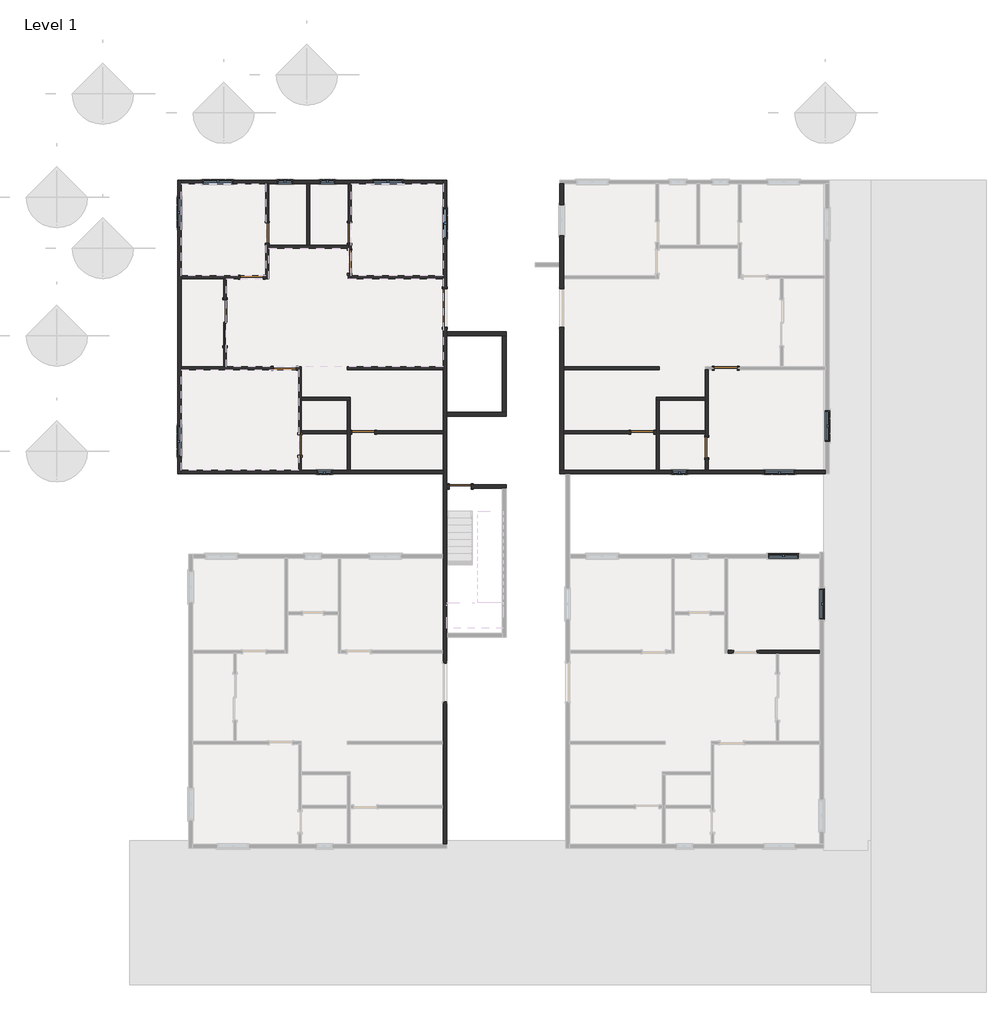
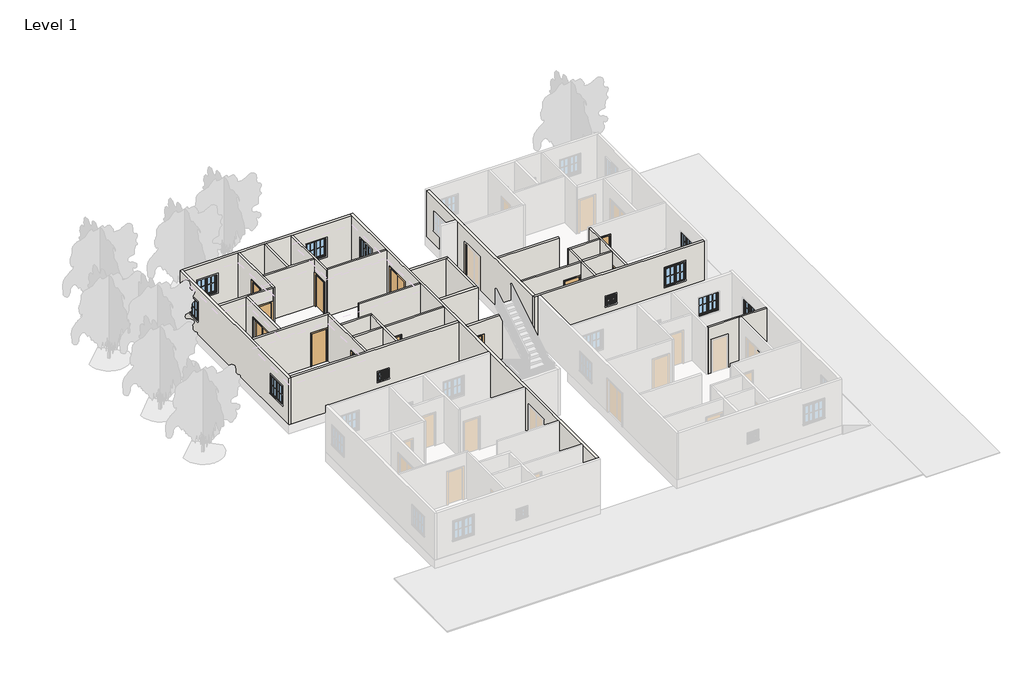
# One storey, part 2 of 7: 29 walls, 13 doors, 13 windows.
"""IFC4 building model written with IfcOpenShell, lengths in millimetres."""

from ifc_helpers import new_model, si_unit, frame, origin, origin_with_axes, place, context, project, spatial, polyline, outline, extrude, faceted_brep, transform, mapped, element, save
from components import door_a09c2f77, door_166d4031, door_d141acb4, door_b6e9fca3, door_e5f9f3c4, window_0c121b81, window_191d0cfb

model = new_model("IFC4")

# Units and contexts
model_context = context("Model", 3, world=origin())
ifc_project = project(units=[si_unit("LENGTHUNIT", "METRE", prefix="MILLI")], contexts=[model_context])

# Site, building, storey
site = spatial("IfcSite", under=ifc_project)
building = spatial("IfcBuilding", under=site)
storey = spatial("IfcBuildingStorey", under=building, Name="Level 1", Elevation=0.0)

# Doors
placement = place(None, origin())
door_shape = door_a09c2f77(model_context)
element("IfcDoor", 1, ObjectType="Door-Double-Flush_Panel : 60\" x 84\"", at=placement, inside=storey, context=model_context, shape_type="MappedRepresentation", body=[
    mapped(door_shape, transform((-3579.3844485, 8733.602842, 0.0), x_axis=(0.0, 1.0, 0.0), y_axis=(-1.0, 0.0, 0.0), z_axis=(0.0, 0.0, 1.0))),
])
door_2_shape = door_166d4031(model_context)
element("IfcDoor", 2, ObjectType="Door-Double-Sliding : 72\" x 84\"", at=placement, inside=storey, context=model_context, shape_type="MappedRepresentation", body=[
    mapped(door_2_shape, transform((-12450.3344485, 8145.4935985, 0.0), x_axis=(0.0, -1.0, 0.0), y_axis=(1.0, 0.0, 0.0), z_axis=(0.0, 0.0, 1.0))),
])
door_3_shape = door_d141acb4(model_context)
element("IfcDoor", 3, ObjectType="Single-Flush : 32\" x 84\"", at=placement, inside=storey, context=model_context, shape_type="MappedRepresentation", body=[
    mapped(door_3_shape, transform((-10646.9344485, 11707.8435985, 0.0), x_axis=(0.0, -1.0, 0.0), y_axis=(1.0, 0.0, 0.0), z_axis=(0.0, 0.0, 1.0))),
])
element("IfcDoor", 4, ObjectType="Single-Flush : 32\" x 84\"", at=placement, inside=storey, context=model_context, shape_type="MappedRepresentation", body=[
    mapped(door_3_shape, transform((-7370.3344485, 11707.8435985, 0.0), x_axis=(0.0, 1.0, 0.0), y_axis=(-1.0, 0.0, 0.0), z_axis=(0.0, 0.0, 1.0))),
])
element("IfcDoor", 5, ObjectType="Single-Flush : 32\" x 84\"", at=placement, inside=storey, context=model_context, shape_type="MappedRepresentation", body=[
    mapped(door_3_shape, transform((-9338.8344485, 3287.7435985, 0.0), x_axis=(0.0, -1.0, 0.0), y_axis=(1.0, 0.0, 0.0), z_axis=(0.0, 0.0, 1.0))),
])
element("IfcDoor", 6, ObjectType="Single-Flush : 32\" x 84\"", at=placement, inside=storey, context=model_context, shape_type="MappedRepresentation", body=[
    mapped(door_3_shape, transform((6828.3514317, 3186.1435985, 0.0), x_axis=(0.0, 1.0, 0.0), y_axis=(-1.0, 0.0, 0.0), z_axis=(0.0, 0.0, 1.0))),
])
door_4_shape = door_b6e9fca3(model_context)
element("IfcDoor", 7, ObjectType="Single-Flush : 34\" x 84\"", at=placement, inside=storey, context=model_context, shape_type="MappedRepresentation", body=[
    mapped(door_4_shape, transform((-2969.7844485, 1636.9269271, 0.0), x_axis=(1.0, 0.0, 0.0), y_axis=(0.0, 1.0, 0.0), z_axis=(0.0, 0.0, 1.0))),
])
door_5_shape = door_e5f9f3c4(model_context)
element("IfcDoor", 8, ObjectType="Single-Flush : 36\" x 84\"", at=placement, inside=storey, context=model_context, shape_type="MappedRepresentation", body=[
    mapped(door_5_shape, transform((-11256.5344485, 9955.2435985, 0.0), x_axis=(1.0, 0.0, 0.0), y_axis=(0.0, 1.0, 0.0), z_axis=(0.0, 0.0, 1.0))),
])
element("IfcDoor", 9, ObjectType="Single-Flush : 36\" x 84\"", at=placement, inside=storey, context=model_context, shape_type="MappedRepresentation", body=[
    mapped(door_5_shape, transform((-7370.3344485, 10564.8435985, 0.0), x_axis=(0.0, -1.0, 0.0), y_axis=(1.0, 0.0, 0.0), z_axis=(0.0, 0.0, 1.0))),
])
element("IfcDoor", 10, ObjectType="Single-Flush : 36\" x 84\"", at=placement, inside=storey, context=model_context, shape_type="MappedRepresentation", body=[
    mapped(door_5_shape, transform((-9948.4344485, 6335.7435985, 0.0), x_axis=(-1.0, 0.0, 0.0), y_axis=(0.0, -1.0, 0.0), z_axis=(0.0, 0.0, 1.0))),
])
element("IfcDoor", 11, ObjectType="Single-Flush : 36\" x 84\"", at=placement, inside=storey, context=model_context, shape_type="MappedRepresentation", body=[
    mapped(door_5_shape, transform((-6824.2344485, 3795.7435985, 0.0), x_axis=(1.0, 0.0, 0.0), y_axis=(0.0, 1.0, 0.0), z_axis=(0.0, 0.0, 1.0))),
])
element("IfcDoor", 12, ObjectType="Single-Flush : 36\" x 84\"", at=placement, inside=storey, context=model_context, shape_type="MappedRepresentation", body=[
    mapped(door_5_shape, transform((7590.3514317, 6335.7435985, 0.0), x_axis=(1.0, 0.0, 0.0), y_axis=(0.0, 1.0, 0.0), z_axis=(0.0, 0.0, 1.0))),
])
element("IfcDoor", 13, ObjectType="Single-Flush : 36\" x 84\"", at=placement, inside=storey, context=model_context, shape_type="MappedRepresentation", body=[
    mapped(door_5_shape, transform((4262.9514317, 3795.7435985, 0.0), x_axis=(1.0, 0.0, 0.0), y_axis=(0.0, 1.0, 0.0), z_axis=(0.0, 0.0, 1.0))),
])

# Walls
element("IfcWall", 14, ObjectType="4.5\"", at=placement, inside=storey, context=model_context, shape_type="Brep", body=[
    faceted_brep([(-10704.0844485, 11301.4435985, 2133.6), (-10704.0844485, 11301.4435985, 0.0), (-10704.0844485, 10012.3935985, 0.0), (-10704.0844485, 9898.0935985, 0.0), (-10704.0844485, 9898.0935985, 3048.0), (-10704.0844485, 10012.3935985, 3048.0), (-10704.0844485, 13669.9935985, 3048.0), (-10704.0844485, 13669.9935985, 0.0), (-10704.0844485, 12114.2435985, 0.0), (-10704.0844485, 12114.2435985, 2133.6), (-10589.7844485, 9898.0935985, 0.0), (-10589.7844485, 11117.2935985, 0.0), (-10589.7844485, 11231.5935985, 0.0), (-10589.7844485, 11301.4435985, 0.0), (-10589.7844485, 11301.4435985, 2133.6), (-10589.7844485, 12114.2435985, 2133.6), (-10589.7844485, 12114.2435985, 0.0), (-10589.7844485, 13669.9935985, 0.0), (-10589.7844485, 13669.9935985, 3048.0), (-10589.7844485, 11231.5935985, 3048.0), (-10589.7844485, 11117.2935985, 3048.0), (-10589.7844485, 9898.0935985, 3048.0)], [[[0, 1, 2, 3, 4, 5, 6, 7, 8, 9]], [[10, 11, 12, 13, 14, 15, 16, 17, 18, 19, 20, 21]], [[8, 7, 17, 16]], [[3, 2, 1, 13, 12, 11, 10]], [[7, 6, 18, 17]], [[4, 3, 10, 21]], [[14, 13, 1, 0]], [[15, 14, 0, 9]], [[16, 15, 9, 8]], [[6, 5, 4, 21, 20, 19, 18]]]),
])
element("IfcWall", 15, ObjectType="4.5\"", at=placement, inside=storey, context=model_context, shape_type="Brep", body=[
    faceted_brep([(-10704.0844485, 10012.3935985, 0.0), (-10799.3344485, 10012.3935985, 0.0), (-10799.3344485, 10012.3935985, 2133.6), (-11713.7344485, 10012.3935985, 2133.6), (-11713.7344485, 10012.3935985, 0.0), (-14056.8844485, 10012.3935985, 0.0), (-14056.8844485, 10012.3935985, 3048.0), (-10704.0844485, 10012.3935985, 3048.0), (-10799.3344485, 9898.0935985, 2133.6), (-10799.3344485, 9898.0935985, 0.0), (-10704.0844485, 9898.0935985, 0.0), (-10704.0844485, 9898.0935985, 3048.0), (-12266.1844485, 9898.0935985, 3048.0), (-12380.4844485, 9898.0935985, 3048.0), (-14056.8844485, 9898.0935985, 3048.0), (-14056.8844485, 9898.0935985, 0.0), (-12380.4844485, 9898.0935985, 0.0), (-12266.1844485, 9898.0935985, 0.0), (-11713.7344485, 9898.0935985, 0.0), (-11713.7344485, 9898.0935985, 2133.6)], [[[0, 1, 2, 3, 4, 5, 6, 7]], [[8, 9, 10, 11, 12, 13, 14, 15, 16, 17, 18, 19]], [[10, 9, 1, 0]], [[18, 17, 16, 15, 5, 4]], [[0, 7, 11, 10]], [[6, 5, 15, 14]], [[2, 1, 9, 8]], [[3, 2, 8, 19]], [[4, 3, 19, 18]], [[7, 6, 14, 13, 12, 11]]]),
])
element("IfcWall", 16, ObjectType="4.5\"", at=placement, inside=storey, context=model_context, shape_type="Brep", body=[
    faceted_brep([(-10589.7844485, 11117.2935985, 0.0), (-7427.4844485, 11117.2935985, 0.0), (-7427.4844485, 11117.2935985, 3048.0), (-10589.7844485, 11117.2935985, 3048.0), (-10589.7844485, 11231.5935985, 0.0), (-10589.7844485, 11231.5935985, 3048.0), (-9065.7844485, 11231.5935985, 3048.0), (-8951.4844485, 11231.5935985, 3048.0), (-7427.4844485, 11231.5935985, 3048.0), (-7427.4844485, 11231.5935985, 0.0), (-8951.4844485, 11231.5935985, 0.0), (-9065.7844485, 11231.5935985, 0.0)], [[[0, 1, 2, 3]], [[4, 5, 6, 7, 8, 9, 10, 11]], [[1, 0, 4, 11, 10, 9]], [[0, 3, 5, 4]], [[2, 1, 9, 8]], [[3, 2, 8, 7, 6, 5]]]),
])
element("IfcWall", 17, ObjectType="4.5\"", at=placement, inside=storey, context=model_context, shape_type="SweptSolid", body=[
    extrude(outline(polyline([(-9065.7844485, 11231.5935985), (-9065.7844485, 13669.9935985), (-8951.4844485, 13669.9935985), (-8951.4844485, 11231.5935985), (-9065.7844485, 11231.5935985)])), origin_with_axes(), (0.0, 0.0, 1.0), 3048.0),
])
element("IfcWall", 18, ObjectType="4.5\"", at=placement, inside=storey, context=model_context, shape_type="Brep", body=[
    faceted_brep([(-7427.4844485, 13669.9935985, 0.0), (-7427.4844485, 12114.2435985, 0.0), (-7427.4844485, 12114.2435985, 2133.6), (-7427.4844485, 11301.4435985, 2133.6), (-7427.4844485, 11301.4435985, 0.0), (-7427.4844485, 11231.5935985, 0.0), (-7427.4844485, 11117.2935985, 0.0), (-7427.4844485, 11022.0435985, 0.0), (-7427.4844485, 11022.0435985, 2133.6), (-7427.4844485, 10107.6435985, 2133.6), (-7427.4844485, 10107.6435985, 0.0), (-7427.4844485, 9898.0935985, 0.0), (-7427.4844485, 9898.0935985, 3048.0), (-7427.4844485, 11117.2935985, 3048.0), (-7427.4844485, 11231.5935985, 3048.0), (-7427.4844485, 13669.9935985, 3048.0), (-7313.1844485, 12114.2435985, 2133.6), (-7313.1844485, 12114.2435985, 0.0), (-7313.1844485, 13669.9935985, 0.0), (-7313.1844485, 13669.9935985, 3048.0), (-7313.1844485, 10012.3935985, 3048.0), (-7313.1844485, 9898.0935985, 3048.0), (-7313.1844485, 9898.0935985, 0.0), (-7313.1844485, 10012.3935985, 0.0), (-7313.1844485, 10107.6435985, 0.0), (-7313.1844485, 10107.6435985, 2133.6), (-7313.1844485, 11022.0435985, 2133.6), (-7313.1844485, 11022.0435985, 0.0), (-7313.1844485, 11301.4435985, 0.0), (-7313.1844485, 11301.4435985, 2133.6)], [[[0, 1, 2, 3, 4, 5, 6, 7, 8, 9, 10, 11, 12, 13, 14, 15]], [[16, 17, 18, 19, 20, 21, 22, 23, 24, 25, 26, 27, 28, 29]], [[11, 10, 24, 23, 22]], [[28, 27, 7, 6, 5, 4]], [[18, 17, 1, 0]], [[0, 15, 19, 18]], [[12, 11, 22, 21]], [[25, 24, 10, 9]], [[26, 25, 9, 8]], [[27, 26, 8, 7]], [[2, 1, 17, 16]], [[3, 2, 16, 29]], [[4, 3, 29, 28]], [[15, 14, 13, 12, 21, 20, 19]]]),
])
element("IfcWall", 19, ObjectType="4.5\"", at=placement, inside=storey, context=model_context, shape_type="SweptSolid", body=[
    extrude(outline(polyline([(-3655.5844485, 9898.0935985), (-7313.1844485, 9898.0935985), (-7313.1844485, 10012.3935985), (-3655.5844485, 10012.3935985), (-3655.5844485, 9898.0935985)])), origin_with_axes(), (0.0, 0.0, 1.0), 3048.0),
])
element("IfcWall", 20, ObjectType="4.5\"", at=placement, inside=storey, context=model_context, shape_type="SweptSolid", body=[
    extrude(outline(polyline([(7231.0935985, 2133.6), (7231.0935985, 0.0), (6392.8935985, 0.0), (6392.8935985, 3048.0), (9898.0935985, 3048.0), (9898.0935985, 0.0), (9059.8935985, 0.0), (9059.8935985, 2133.6), (7231.0935985, 2133.6)])), frame((-12380.4844485, 0.0, 0.0), z_axis=(1.0, 0.0, 0.0), x_axis=(0.0, 1.0, 0.0)), (0.0, 0.0, 1.0), 114.3),
])
element("IfcWall", 21, ObjectType="4.5\"", at=placement, inside=storey, context=model_context, shape_type="Brep", body=[
    faceted_brep([(-14056.8844485, 6278.5935985, 0.0), (-10405.6344485, 6278.5935985, 0.0), (-10405.6344485, 6278.5935985, 2133.6), (-9491.2344485, 6278.5935985, 2133.6), (-9491.2344485, 6278.5935985, 0.0), (-9395.9844485, 6278.5935985, 0.0), (-9281.6844485, 6278.5935985, 0.0), (-9281.6844485, 6278.5935985, 3048.0), (-9395.9844485, 6278.5935985, 3048.0), (-14056.8844485, 6278.5935985, 3048.0), (-10405.6344485, 6392.8935985, 2133.6), (-10405.6344485, 6392.8935985, 0.0), (-12266.1844485, 6392.8935985, 0.0), (-12380.4844485, 6392.8935985, 0.0), (-14056.8844485, 6392.8935985, 0.0), (-14056.8844485, 6392.8935985, 3048.0), (-12380.4844485, 6392.8935985, 3048.0), (-12266.1844485, 6392.8935985, 3048.0), (-9281.6844485, 6392.8935985, 3048.0), (-9281.6844485, 6392.8935985, 0.0), (-9491.2344485, 6392.8935985, 0.0), (-9491.2344485, 6392.8935985, 2133.6)], [[[0, 1, 2, 3, 4, 5, 6, 7, 8, 9]], [[10, 11, 12, 13, 14, 15, 16, 17, 18, 19, 20, 21]], [[20, 19, 6, 5, 4]], [[14, 13, 12, 11, 1, 0]], [[0, 9, 15, 14]], [[7, 6, 19, 18]], [[2, 1, 11, 10]], [[3, 2, 10, 21]], [[4, 3, 21, 20]], [[9, 8, 7, 18, 17, 16, 15]]]),
])
element("IfcWall", 22, ObjectType="4.5\"", at=placement, inside=storey, context=model_context, shape_type="Brep", body=[
    faceted_brep([(-9395.9844485, 2881.3435985, 2133.6), (-9395.9844485, 2881.3435985, 0.0), (-9395.9844485, 2290.7935985, 0.0), (-9395.9844485, 2290.7935985, 3048.0), (-9395.9844485, 6278.5935985, 3048.0), (-9395.9844485, 6278.5935985, 0.0), (-9395.9844485, 3694.1435985, 0.0), (-9395.9844485, 3694.1435985, 2133.6), (-9281.6844485, 2290.7935985, 0.0), (-9281.6844485, 2881.3435985, 0.0), (-9281.6844485, 2881.3435985, 2133.6), (-9281.6844485, 3694.1435985, 2133.6), (-9281.6844485, 3694.1435985, 0.0), (-9281.6844485, 3738.5935985, 0.0), (-9281.6844485, 3852.8935985, 0.0), (-9281.6844485, 5072.0935985, 0.0), (-9281.6844485, 5186.3935985, 0.0), (-9281.6844485, 6278.5935985, 0.0), (-9281.6844485, 6278.5935985, 3048.0), (-9281.6844485, 5186.3935985, 3048.0), (-9281.6844485, 5072.0935985, 3048.0), (-9281.6844485, 3852.8935985, 3048.0), (-9281.6844485, 3738.5935985, 3048.0), (-9281.6844485, 2290.7935985, 3048.0)], [[[0, 1, 2, 3, 4, 5, 6, 7]], [[8, 9, 10, 11, 12, 13, 14, 15, 16, 17, 18, 19, 20, 21, 22, 23]], [[6, 5, 17, 16, 15, 14, 13, 12]], [[2, 1, 9, 8]], [[5, 4, 18, 17]], [[3, 2, 8, 23]], [[10, 9, 1, 0]], [[11, 10, 0, 7]], [[12, 11, 7, 6]], [[4, 3, 23, 22, 21, 20, 19, 18]]]),
])
element("IfcWall", 23, ObjectType="4.5\"", at=placement, inside=storey, context=model_context, shape_type="Brep", body=[
    faceted_brep([(-9281.6844485, 5072.0935985, 0.0), (-7452.8844485, 5072.0935985, 0.0), (-7338.5844485, 5072.0935985, 0.0), (-7338.5844485, 5072.0935985, 3048.0), (-7452.8844485, 5072.0935985, 3048.0), (-9281.6844485, 5072.0935985, 3048.0), (-9281.6844485, 5186.3935985, 0.0), (-9281.6844485, 5186.3935985, 3048.0), (-7338.5844485, 5186.3935985, 3048.0), (-7338.5844485, 5186.3935985, 0.0)], [[[0, 1, 2, 3, 4, 5]], [[6, 7, 8, 9]], [[2, 1, 0, 6, 9]], [[0, 5, 7, 6]], [[3, 2, 9, 8]], [[5, 4, 3, 8, 7]]]),
])
element("IfcWall", 24, ObjectType="4.5\"", at=placement, inside=storey, context=model_context, shape_type="Brep", body=[
    faceted_brep([(-7452.8844485, 5072.0935985, 0.0), (-7452.8844485, 3852.8935985, 0.0), (-7452.8844485, 3738.5935985, 0.0), (-7452.8844485, 2290.7935985, 0.0), (-7452.8844485, 2290.7935985, 3048.0), (-7452.8844485, 3738.5935985, 3048.0), (-7452.8844485, 3852.8935985, 3048.0), (-7452.8844485, 5072.0935985, 3048.0), (-7338.5844485, 5072.0935985, 0.0), (-7338.5844485, 5072.0935985, 3048.0), (-7338.5844485, 3852.8935985, 3048.0), (-7338.5844485, 3738.5935985, 3048.0), (-7338.5844485, 2290.7935985, 3048.0), (-7338.5844485, 2290.7935985, 0.0), (-7338.5844485, 3738.5935985, 0.0), (-7338.5844485, 3852.8935985, 0.0)], [[[0, 1, 2, 3, 4, 5, 6, 7]], [[8, 9, 10, 11, 12, 13, 14, 15]], [[3, 2, 1, 0, 8, 15, 14, 13]], [[0, 7, 9, 8]], [[4, 3, 13, 12]], [[7, 6, 5, 4, 12, 11, 10, 9]]]),
])
element("IfcWall", 25, ObjectType="4.5\"", at=placement, inside=storey, context=model_context, shape_type="SweptSolid", body=[
    extrude(outline(polyline([(-9281.6844485, 3738.5935985), (-9281.6844485, 3852.8935985), (-7452.8844485, 3852.8935985), (-7452.8844485, 3738.5935985), (-9281.6844485, 3738.5935985)])), origin_with_axes(), (0.0, 0.0, 1.0), 3048.0),
    extrude(outline(polyline([(0.0, -3655.5844485), (3048.0, -3655.5844485), (3048.0, -7338.5844485), (0.0, -7338.5844485), (0.0, -7281.4344485), (2133.6, -7281.4344485), (2133.6, -6367.0344485), (0.0, -6367.0344485), (0.0, -3655.5844485)])), frame((0.0, 3738.5935985, 0.0), z_axis=(0.0, 1.0, 0.0), x_axis=(0.0, 0.0, 1.0)), (0.0, 0.0, 1.0), 114.3),
])
element("IfcWall", 26, ObjectType="4.5\"", at=placement, inside=storey, context=model_context, shape_type="SweptSolid", body=[
    extrude(outline(polyline([(-3655.5844485, 6278.5935985), (-7452.8844485, 6278.5935985), (-7452.8844485, 6392.8935985), (-3655.5844485, 6392.8935985), (-3655.5844485, 6278.5935985)])), origin_with_axes(), (0.0, 0.0, 1.0), 3048.0),
])
element("IfcWall", 27, ObjectType="4.5\"", at=placement, inside=storey, context=model_context, shape_type="Brep", body=[
    faceted_brep([(6771.2014317, 6278.5935985, 0.0), (6771.2014317, 5186.3935985, 0.0), (6771.2014317, 5072.0935985, 0.0), (6771.2014317, 3852.8935985, 0.0), (6771.2014317, 3738.5935985, 0.0), (6771.2014317, 3592.5435985, 0.0), (6771.2014317, 3592.5435985, 2133.6), (6771.2014317, 2779.7435985, 2133.6), (6771.2014317, 2779.7435985, 0.0), (6771.2014317, 2290.7935985, 0.0), (6771.2014317, 2290.7935985, 3048.0), (6771.2014317, 3738.5935985, 3048.0), (6771.2014317, 3852.8935985, 3048.0), (6771.2014317, 5072.0935985, 3048.0), (6771.2014317, 5186.3935985, 3048.0), (6771.2014317, 6278.5935985, 3048.0), (6885.5014317, 3592.5435985, 2133.6), (6885.5014317, 3592.5435985, 0.0), (6885.5014317, 6278.5935985, 0.0), (6885.5014317, 6278.5935985, 3048.0), (6885.5014317, 2290.7935985, 3048.0), (6885.5014317, 2290.7935985, 0.0), (6885.5014317, 2779.7435985, 0.0), (6885.5014317, 2779.7435985, 2133.6)], [[[0, 1, 2, 3, 4, 5, 6, 7, 8, 9, 10, 11, 12, 13, 14, 15]], [[16, 17, 18, 19, 20, 21, 22, 23]], [[22, 21, 9, 8]], [[18, 17, 5, 4, 3, 2, 1, 0]], [[0, 15, 19, 18]], [[10, 9, 21, 20]], [[6, 5, 17, 16]], [[7, 6, 16, 23]], [[8, 7, 23, 22]], [[15, 14, 13, 12, 11, 10, 20, 19]]]),
])
element("IfcWall", 28, ObjectType="4.5\"", at=placement, inside=storey, context=model_context, shape_type="Brep", body=[
    faceted_brep([(6771.2014317, 5186.3935985, 0.0), (4828.1014317, 5186.3935985, 0.0), (4828.1014317, 5186.3935985, 3048.0), (6771.2014317, 5186.3935985, 3048.0), (6771.2014317, 5072.0935985, 0.0), (6771.2014317, 5072.0935985, 3048.0), (4942.4014317, 5072.0935985, 3048.0), (4828.1014317, 5072.0935985, 3048.0), (4828.1014317, 5072.0935985, 0.0), (4942.4014317, 5072.0935985, 0.0)], [[[0, 1, 2, 3]], [[4, 5, 6, 7, 8, 9]], [[1, 0, 4, 9, 8]], [[0, 3, 5, 4]], [[2, 1, 8, 7]], [[3, 2, 7, 6, 5]]]),
])
element("IfcWall", 29, ObjectType="4.5\"", at=placement, inside=storey, context=model_context, shape_type="Brep", body=[
    faceted_brep([(4828.1014317, 5072.0935985, 0.0), (4828.1014317, 3852.8935985, 0.0), (4828.1014317, 3738.5935985, 0.0), (4828.1014317, 2290.7935985, 0.0), (4828.1014317, 2290.7935985, 3048.0), (4828.1014317, 3738.5935985, 3048.0), (4828.1014317, 3852.8935985, 3048.0), (4828.1014317, 5072.0935985, 3048.0), (4942.4014317, 5072.0935985, 0.0), (4942.4014317, 5072.0935985, 3048.0), (4942.4014317, 3852.8935985, 3048.0), (4942.4014317, 3738.5935985, 3048.0), (4942.4014317, 2290.7935985, 3048.0), (4942.4014317, 2290.7935985, 0.0), (4942.4014317, 3738.5935985, 0.0), (4942.4014317, 3852.8935985, 0.0)], [[[0, 1, 2, 3, 4, 5, 6, 7]], [[8, 9, 10, 11, 12, 13, 14, 15]], [[3, 2, 1, 0, 8, 15, 14, 13]], [[0, 7, 9, 8]], [[4, 3, 13, 12]], [[7, 6, 5, 4, 12, 11, 10, 9]]]),
])
element("IfcWall", 30, ObjectType="4.5\"", at=placement, inside=storey, context=model_context, shape_type="SweptSolid", body=[
    extrude(outline(polyline([(3048.0, 1145.1014317), (0.0, 1145.1014317), (0.0, 3805.7514317), (2133.6, 3805.7514317), (2133.6, 4720.1514317), (0.0, 4720.1514317), (0.0, 4828.1014317), (3048.0, 4828.1014317), (3048.0, 1145.1014317)])), frame((0.0, 3738.5935985, 0.0), z_axis=(0.0, 1.0, 0.0), x_axis=(0.0, 0.0, 1.0)), (0.0, 0.0, 1.0), 114.3),
    extrude(outline(polyline([(6771.2014317, 3852.8935985), (6771.2014317, 3738.5935985), (4942.4014317, 3738.5935985), (4942.4014317, 3852.8935985), (6771.2014317, 3852.8935985)])), origin_with_axes(), (0.0, 0.0, 1.0), 3048.0),
])
element("IfcWall", 31, ObjectType="4.5\"", at=placement, inside=storey, context=model_context, shape_type="SweptSolid", body=[
    extrude(outline(polyline([(4942.4014317, 6278.5935985), (1145.1014317, 6278.5935985), (1145.1014317, 6392.8935985), (4942.4014317, 6392.8935985), (4942.4014317, 6278.5935985)])), origin_with_axes(), (0.0, 0.0, 1.0), 3048.0),
])
element("IfcWall", 32, ObjectType="4.5\"", at=placement, inside=storey, context=model_context, shape_type="Brep", body=[
    faceted_brep([(7665.1785285, -4986.3064015, 0.0), (7912.8285285, -4986.3064015, 0.0), (7912.8285285, -4986.3064015, 2133.6), (8827.2285285, -4986.3064015, 2133.6), (8827.2285285, -4986.3064015, 0.0), (9584.1655515, -4986.3064015, 0.0), (9698.4655515, -4986.3064015, 0.0), (11322.7785285, -4986.3064015, 0.0), (11322.7785285, -4986.3064015, 3048.0), (9698.4655515, -4986.3064015, 3048.0), (9584.1655515, -4986.3064015, 3048.0), (7665.1785285, -4986.3064015, 3048.0), (7912.8285285, -4872.0064015, 2133.6), (7912.8285285, -4872.0064015, 0.0), (7665.1785285, -4872.0064015, 0.0), (7665.1785285, -4872.0064015, 3048.0), (11322.7785285, -4872.0064015, 3048.0), (11322.7785285, -4872.0064015, 0.0), (8827.2285285, -4872.0064015, 0.0), (8827.2285285, -4872.0064015, 2133.6)], [[[0, 1, 2, 3, 4, 5, 6, 7, 8, 9, 10, 11]], [[12, 13, 14, 15, 16, 17, 18, 19]], [[18, 17, 7, 6, 5, 4]], [[14, 13, 1, 0]], [[0, 11, 15, 14]], [[8, 7, 17, 16]], [[2, 1, 13, 12]], [[3, 2, 12, 19]], [[4, 3, 19, 18]], [[11, 10, 9, 8, 16, 15]]]),
])
element("IfcWall", 33, ObjectType="6\"", at=placement, inside=storey, context=model_context, shape_type="Brep", body=[
    faceted_brep([(-14209.2844485, 13822.3935985, 0.0), (-14209.2844485, 2138.3935985, 0.0), (-14209.2844485, 2138.3935985, 3048.0), (-14209.2844485, 13822.3935985, 3048.0), (-14209.2844485, 13136.5935985, 2133.6), (-14209.2844485, 11917.3935985, 2133.6), (-14209.2844485, 11917.3935985, 914.4), (-14209.2844485, 13136.5935985, 914.4), (-14209.2844485, 4043.3935985, 2133.6), (-14209.2844485, 2824.1935985, 2133.6), (-14209.2844485, 2824.1935985, 914.4), (-14209.2844485, 4043.3935985, 914.4), (-14056.8844485, 13822.3935985, 0.0), (-14056.8844485, 13822.3935985, 3048.0), (-14056.8844485, 13669.9935985, 3048.0), (-14056.8844485, 10012.3935985, 3048.0), (-14056.8844485, 9898.0935985, 3048.0), (-14056.8844485, 6392.8935985, 3048.0), (-14056.8844485, 6278.5935985, 3048.0), (-14056.8844485, 2290.7935985, 3048.0), (-14056.8844485, 2138.3935985, 3048.0), (-14056.8844485, 2138.3935985, 0.0), (-14056.8844485, 2290.7935985, 0.0), (-14056.8844485, 6278.5935985, 0.0), (-14056.8844485, 6392.8935985, 0.0), (-14056.8844485, 9898.0935985, 0.0), (-14056.8844485, 10012.3935985, 0.0), (-14056.8844485, 13669.9935985, 0.0), (-14056.8844485, 13136.5935985, 2133.6), (-14056.8844485, 13136.5935985, 914.4), (-14056.8844485, 11917.3935985, 914.4), (-14056.8844485, 11917.3935985, 2133.6), (-14056.8844485, 4043.3935985, 2133.6), (-14056.8844485, 4043.3935985, 914.4), (-14056.8844485, 2824.1935985, 914.4), (-14056.8844485, 2824.1935985, 2133.6)], [[[0, 1, 2, 3], [4, 5, 6, 7], [8, 9, 10, 11]], [[12, 13, 14, 15, 16, 17, 18, 19, 20, 21, 22, 23, 24, 25, 26, 27], [28, 29, 30, 31], [32, 33, 34, 35]], [[1, 0, 12, 27, 26, 25, 24, 23, 22, 21]], [[2, 1, 21, 20]], [[0, 3, 13, 12]], [[29, 28, 4, 7]], [[30, 29, 7, 6]], [[31, 30, 6, 5]], [[28, 31, 5, 4]], [[33, 32, 8, 11]], [[34, 33, 11, 10]], [[35, 34, 10, 9]], [[32, 35, 9, 8]], [[3, 2, 20, 19, 18, 17, 16, 15, 14, 13]]]),
])
element("IfcWall", 34, ObjectType="6\"", at=placement, inside=storey, context=model_context, shape_type="Brep", body=[
    faceted_brep([(-14056.8844485, 2138.3935985, 0.0), (-3655.5844485, 2138.3935985, 0.0), (-3655.5844485, 2138.3935985, 3048.0), (-14056.8844485, 2138.3935985, 3048.0), (-8672.0844485, 2138.3935985, 1524.0), (-8062.4844485, 2138.3935985, 1524.0), (-8062.4844485, 2138.3935985, 914.4), (-8672.0844485, 2138.3935985, 914.4), (-14056.8844485, 2290.7935985, 0.0), (-14056.8844485, 2290.7935985, 3048.0), (-9395.9844485, 2290.7935985, 3048.0), (-9281.6844485, 2290.7935985, 3048.0), (-7452.8844485, 2290.7935985, 3048.0), (-7338.5844485, 2290.7935985, 3048.0), (-3655.5844485, 2290.7935985, 3048.0), (-3655.5844485, 2290.7935985, 0.0), (-7338.5844485, 2290.7935985, 0.0), (-7452.8844485, 2290.7935985, 0.0), (-9281.6844485, 2290.7935985, 0.0), (-9395.9844485, 2290.7935985, 0.0), (-8672.0844485, 2290.7935985, 1524.0), (-8672.0844485, 2290.7935985, 914.4), (-8062.4844485, 2290.7935985, 914.4), (-8062.4844485, 2290.7935985, 1524.0)], [[[0, 1, 2, 3], [4, 5, 6, 7]], [[8, 9, 10, 11, 12, 13, 14, 15, 16, 17, 18, 19], [20, 21, 22, 23]], [[1, 0, 8, 19, 18, 17, 16, 15]], [[0, 3, 9, 8]], [[2, 1, 15, 14]], [[21, 20, 4, 7]], [[22, 21, 7, 6]], [[23, 22, 6, 5]], [[20, 23, 5, 4]], [[3, 2, 14, 13, 12, 11, 10, 9]]]),
])
element("IfcWall", 35, ObjectType="6\"", at=placement, inside=storey, context=model_context, shape_type="Brep", body=[
    faceted_brep([(-3503.1844485, 13822.3935985, 0.0), (-3503.1844485, 13822.3935985, 3048.0), (-3503.1844485, 7791.3620855, 3048.0), (-3503.1844485, 7638.9620855, 3048.0), (-3503.1844485, 4590.9620855, 3048.0), (-3503.1844485, 4438.5620855, 3048.0), (-3503.1844485, 1713.1269271, 3048.0), (-3503.1844485, 1560.7269271, 3048.0), (-3503.1844485, -4001.8730729, 3048.0), (-3503.1844485, -4205.0730729, 3048.0), (-3503.1844485, -4357.4730729, 3048.0), (-3503.1844485, -12593.6064015, 3048.0), (-3503.1844485, -12593.6064015, 0.0), (-3503.1844485, -6910.3564015, 0.0), (-3503.1844485, -6910.3564015, 2133.6), (-3503.1844485, -5386.3564015, 2133.6), (-3503.1844485, -5386.3564015, 0.0), (-3503.1844485, -4357.4730729, 0.0), (-3503.1844485, -4205.0730729, 0.0), (-3503.1844485, 1560.7269271, 0.0), (-3503.1844485, 1713.1269271, 0.0), (-3503.1844485, 4438.5620855, 0.0), (-3503.1844485, 4590.9620855, 0.0), (-3503.1844485, 7638.9620855, 0.0), (-3503.1844485, 7791.3620855, 0.0), (-3503.1844485, 7971.602842, 0.0), (-3503.1844485, 7971.602842, 2133.6), (-3503.1844485, 9495.602842, 2133.6), (-3503.1844485, 9495.602842, 0.0), (-3503.1844485, 11493.4926514, 2133.6), (-3503.1844485, 12712.6926514, 2133.6), (-3503.1844485, 12712.6926514, 914.4), (-3503.1844485, 11493.4926514, 914.4), (-3655.5844485, -12593.6064015, 3048.0), (-3655.5844485, -11145.8064015, 3048.0), (-3655.5844485, -11031.5064015, 3048.0), (-3655.5844485, -8605.8064015, 3048.0), (-3655.5844485, -8491.5064015, 3048.0), (-3655.5844485, -4986.3064015, 3048.0), (-3655.5844485, -4872.0064015, 3048.0), (-3655.5844485, -1214.4064015, 3048.0), (-3655.5844485, -1062.0064015, 3048.0), (-3655.5844485, 2138.3935985, 3048.0), (-3655.5844485, 2290.7935985, 3048.0), (-3655.5844485, 3738.5935985, 3048.0), (-3655.5844485, 3852.8935985, 3048.0), (-3655.5844485, 6278.5935985, 3048.0), (-3655.5844485, 6392.8935985, 3048.0), (-3655.5844485, 9898.0935985, 3048.0), (-3655.5844485, 10012.3935985, 3048.0), (-3655.5844485, 13669.9935985, 3048.0), (-3655.5844485, 13822.3935985, 3048.0), (-3655.5844485, 13822.3935985, 0.0), (-3655.5844485, 13669.9935985, 0.0), (-3655.5844485, 10012.3935985, 0.0), (-3655.5844485, 9898.0935985, 0.0), (-3655.5844485, 9495.602842, 0.0), (-3655.5844485, 9495.602842, 2133.6), (-3655.5844485, 7971.602842, 2133.6), (-3655.5844485, 7971.602842, 0.0), (-3655.5844485, 6392.8935985, 0.0), (-3655.5844485, 6278.5935985, 0.0), (-3655.5844485, 3852.8935985, 0.0), (-3655.5844485, 3738.5935985, 0.0), (-3655.5844485, 2290.7935985, 0.0), (-3655.5844485, 2138.3935985, 0.0), (-3655.5844485, -1062.0064015, 0.0), (-3655.5844485, -1214.4064015, 0.0), (-3655.5844485, -4872.0064015, 0.0), (-3655.5844485, -4986.3064015, 0.0), (-3655.5844485, -5386.3564015, 0.0), (-3655.5844485, -5386.3564015, 2133.6), (-3655.5844485, -6910.3564015, 2133.6), (-3655.5844485, -6910.3564015, 0.0), (-3655.5844485, -8491.5064015, 0.0), (-3655.5844485, -8605.8064015, 0.0), (-3655.5844485, -11031.5064015, 0.0), (-3655.5844485, -11145.8064015, 0.0), (-3655.5844485, -12593.6064015, 0.0), (-3655.5844485, 11493.4926514, 2133.6), (-3655.5844485, 11493.4926514, 914.4), (-3655.5844485, 12712.6926514, 914.4), (-3655.5844485, 12712.6926514, 2133.6)], [[[0, 1, 2, 3, 4, 5, 6, 7, 8, 9, 10, 11, 12, 13, 14, 15, 16, 17, 18, 19, 20, 21, 22, 23, 24, 25, 26, 27, 28], [29, 30, 31, 32]], [[33, 34, 35, 36, 37, 38, 39, 40, 41, 42, 43, 44, 45, 46, 47, 48, 49, 50, 51, 52, 53, 54, 55, 56, 57, 58, 59, 60, 61, 62, 63, 64, 65, 66, 67, 68, 69, 70, 71, 72, 73, 74, 75, 76, 77, 78], [79, 80, 81, 82]], [[52, 0, 28, 56, 55, 54, 53]], [[12, 78, 77, 76, 75, 74, 73, 13]], [[59, 25, 24, 23, 22, 21, 20, 19, 18, 17, 16, 70, 69, 68, 67, 66, 65, 64, 63, 62, 61, 60]], [[1, 0, 52, 51]], [[12, 11, 33, 78]], [[80, 79, 29, 32]], [[81, 80, 32, 31]], [[82, 81, 31, 30]], [[79, 82, 30, 29]], [[27, 57, 56, 28]], [[57, 27, 26, 58]], [[58, 26, 25, 59]], [[15, 71, 70, 16]], [[71, 15, 14, 72]], [[72, 14, 13, 73]], [[51, 50, 49, 48, 47, 46, 45, 44, 43, 42, 41, 40, 39, 38, 37, 36, 35, 34, 33, 11, 10, 9, 8, 7, 6, 5, 4, 3, 2, 1]]]),
])
element("IfcWall", 36, ObjectType="6\"", at=placement, inside=storey, context=model_context, shape_type="Brep", body=[
    faceted_brep([(-3655.5844485, 13822.3935985, 0.0), (-14056.8844485, 13822.3935985, 0.0), (-14056.8844485, 13822.3935985, 3048.0), (-3655.5844485, 13822.3935985, 3048.0), (-11999.4844485, 13822.3935985, 2133.6), (-13218.6844485, 13822.3935985, 2133.6), (-13218.6844485, 13822.3935985, 914.4), (-11999.4844485, 13822.3935985, 914.4), (-5236.7344485, 13822.3935985, 2133.6), (-6455.9344485, 13822.3935985, 2133.6), (-6455.9344485, 13822.3935985, 914.4), (-5236.7344485, 13822.3935985, 914.4), (-9630.9344485, 13822.3935985, 1524.0), (-10240.5344485, 13822.3935985, 1524.0), (-10240.5344485, 13822.3935985, 914.4), (-9630.9344485, 13822.3935985, 914.4), (-7941.8344485, 13822.3935985, 1524.0), (-8551.4344485, 13822.3935985, 1524.0), (-8551.4344485, 13822.3935985, 914.4), (-7941.8344485, 13822.3935985, 914.4), (-3655.5844485, 13669.9935985, 0.0), (-3655.5844485, 13669.9935985, 3048.0), (-7313.1844485, 13669.9935985, 3048.0), (-7427.4844485, 13669.9935985, 3048.0), (-8951.4844485, 13669.9935985, 3048.0), (-9065.7844485, 13669.9935985, 3048.0), (-10589.7844485, 13669.9935985, 3048.0), (-10704.0844485, 13669.9935985, 3048.0), (-14056.8844485, 13669.9935985, 3048.0), (-14056.8844485, 13669.9935985, 0.0), (-10704.0844485, 13669.9935985, 0.0), (-10589.7844485, 13669.9935985, 0.0), (-9065.7844485, 13669.9935985, 0.0), (-8951.4844485, 13669.9935985, 0.0), (-7427.4844485, 13669.9935985, 0.0), (-7313.1844485, 13669.9935985, 0.0), (-11999.4844485, 13669.9935985, 2133.6), (-11999.4844485, 13669.9935985, 914.4), (-13218.6844485, 13669.9935985, 914.4), (-13218.6844485, 13669.9935985, 2133.6), (-5236.7344485, 13669.9935985, 2133.6), (-5236.7344485, 13669.9935985, 914.4), (-6455.9344485, 13669.9935985, 914.4), (-6455.9344485, 13669.9935985, 2133.6), (-9630.9344485, 13669.9935985, 1524.0), (-9630.9344485, 13669.9935985, 914.4), (-10240.5344485, 13669.9935985, 914.4), (-10240.5344485, 13669.9935985, 1524.0), (-7941.8344485, 13669.9935985, 1524.0), (-7941.8344485, 13669.9935985, 914.4), (-8551.4344485, 13669.9935985, 914.4), (-8551.4344485, 13669.9935985, 1524.0)], [[[0, 1, 2, 3], [4, 5, 6, 7], [8, 9, 10, 11], [12, 13, 14, 15], [16, 17, 18, 19]], [[20, 21, 22, 23, 24, 25, 26, 27, 28, 29, 30, 31, 32, 33, 34, 35], [36, 37, 38, 39], [40, 41, 42, 43], [44, 45, 46, 47], [48, 49, 50, 51]], [[1, 0, 20, 35, 34, 33, 32, 31, 30, 29]], [[0, 3, 21, 20]], [[2, 1, 29, 28]], [[37, 36, 4, 7]], [[38, 37, 7, 6]], [[39, 38, 6, 5]], [[36, 39, 5, 4]], [[41, 40, 8, 11]], [[42, 41, 11, 10]], [[43, 42, 10, 9]], [[40, 43, 9, 8]], [[45, 44, 12, 15]], [[46, 45, 15, 14]], [[47, 46, 14, 13]], [[44, 47, 13, 12]], [[49, 48, 16, 19]], [[50, 49, 19, 18]], [[51, 50, 18, 17]], [[48, 51, 17, 16]], [[3, 2, 28, 27, 26, 25, 24, 23, 22, 21]]]),
])
element("IfcWall", 37, ObjectType="6\"", at=placement, inside=storey, context=model_context, shape_type="Brep", body=[
    faceted_brep([(11546.4014317, 2290.7935985, 0.0), (6885.5014317, 2290.7935985, 0.0), (6771.2014317, 2290.7935985, 0.0), (4942.4014317, 2290.7935985, 0.0), (4828.1014317, 2290.7935985, 0.0), (1145.1014317, 2290.7935985, 0.0), (992.7014317, 2290.7935985, 0.0), (992.7014317, 2290.7935985, 3048.0), (1145.1014317, 2290.7935985, 3048.0), (4828.1014317, 2290.7935985, 3048.0), (4942.4014317, 2290.7935985, 3048.0), (6771.2014317, 2290.7935985, 3048.0), (6885.5014317, 2290.7935985, 3048.0), (11546.4014317, 2290.7935985, 3048.0), (9112.9785285, 2290.7935985, 2133.6), (9112.9785285, 2290.7935985, 914.4), (10332.1785285, 2290.7935985, 914.4), (10332.1785285, 2290.7935985, 2133.6), (5444.0514317, 2290.7935985, 1524.0), (5444.0514317, 2290.7935985, 914.4), (6053.6514317, 2290.7935985, 914.4), (6053.6514317, 2290.7935985, 1524.0), (11546.4014317, 2138.3935985, 0.0), (11546.4014317, 2138.3935985, 3048.0), (1373.6155515, 2138.3935985, 3048.0), (1221.2155515, 2138.3935985, 3048.0), (992.7014317, 2138.3935985, 3048.0), (992.7014317, 2138.3935985, 0.0), (1221.2155515, 2138.3935985, 0.0), (1373.6155515, 2138.3935985, 0.0), (9112.9785285, 2138.3935985, 2133.6), (10332.1785285, 2138.3935985, 2133.6), (10332.1785285, 2138.3935985, 914.4), (9112.9785285, 2138.3935985, 914.4), (5444.0514317, 2138.3935985, 1524.0), (6053.6514317, 2138.3935985, 1524.0), (6053.6514317, 2138.3935985, 914.4), (5444.0514317, 2138.3935985, 914.4)], [[[0, 1, 2, 3, 4, 5, 6, 7, 8, 9, 10, 11, 12, 13], [14, 15, 16, 17], [18, 19, 20, 21]], [[22, 23, 24, 25, 26, 27, 28, 29], [30, 31, 32, 33], [34, 35, 36, 37]], [[6, 5, 4, 3, 2, 1, 0, 22, 29, 28, 27]], [[0, 13, 23, 22]], [[7, 6, 27, 26]], [[15, 14, 30, 33]], [[16, 15, 33, 32]], [[17, 16, 32, 31]], [[14, 17, 31, 30]], [[19, 18, 34, 37]], [[20, 19, 37, 36]], [[21, 20, 36, 35]], [[18, 21, 35, 34]], [[13, 12, 11, 10, 9, 8, 7, 26, 25, 24, 23]]]),
])
element("IfcWall", 38, ObjectType="6\"", at=placement, inside=storey, context=model_context, shape_type="Brep", body=[
    faceted_brep([(1145.1014317, 2290.7935985, 3048.0), (1145.1014317, 2290.7935985, 0.0), (1145.1014317, 3738.5935985, 0.0), (1145.1014317, 3852.8935985, 0.0), (1145.1014317, 6278.5935985, 0.0), (1145.1014317, 6392.8935985, 0.0), (1145.1014317, 7974.0435985, 0.0), (1145.1014317, 7974.0435985, 2133.6), (1145.1014317, 9498.0435985, 2133.6), (1145.1014317, 9498.0435985, 0.0), (1145.1014317, 9898.0935985, 0.0), (1145.1014317, 10012.3935985, 0.0), (1145.1014317, 13669.9935985, 0.0), (1145.1014317, 13669.9935985, 3048.0), (1145.1014317, 10012.3935985, 3048.0), (1145.1014317, 9898.0935985, 3048.0), (1145.1014317, 6392.8935985, 3048.0), (1145.1014317, 6278.5935985, 3048.0), (1145.1014317, 3852.8935985, 3048.0), (1145.1014317, 3738.5935985, 3048.0), (1145.1014317, 12831.7935985, 2133.6), (1145.1014317, 12831.7935985, 914.4), (1145.1014317, 11612.5935985, 914.4), (1145.1014317, 11612.5935985, 2133.6), (992.7014317, 2290.7935985, 0.0), (992.7014317, 2290.7935985, 3048.0), (992.7014317, 10383.7917043, 3048.0), (992.7014317, 10536.1917043, 3048.0), (992.7014317, 13669.9935985, 3048.0), (992.7014317, 13669.9935985, 0.0), (992.7014317, 10536.1917043, 0.0), (992.7014317, 10383.7917043, 0.0), (992.7014317, 9498.0435985, 0.0), (992.7014317, 9498.0435985, 2133.6), (992.7014317, 7974.0435985, 2133.6), (992.7014317, 7974.0435985, 0.0), (992.7014317, 12831.7935985, 2133.6), (992.7014317, 11612.5935985, 2133.6), (992.7014317, 11612.5935985, 914.4), (992.7014317, 12831.7935985, 914.4)], [[[0, 1, 2, 3, 4, 5, 6, 7, 8, 9, 10, 11, 12, 13, 14, 15, 16, 17, 18, 19], [20, 21, 22, 23]], [[24, 25, 26, 27, 28, 29, 30, 31, 32, 33, 34, 35], [36, 37, 38, 39]], [[1, 24, 35, 6, 5, 4, 3, 2]], [[29, 12, 11, 10, 9, 32, 31, 30]], [[1, 0, 25, 24]], [[13, 12, 29, 28]], [[21, 20, 36, 39]], [[22, 21, 39, 38]], [[23, 22, 38, 37]], [[20, 23, 37, 36]], [[34, 7, 6, 35]], [[7, 34, 33, 8]], [[8, 33, 32, 9]], [[0, 19, 18, 17, 16, 15, 14, 13, 28, 27, 26, 25]]]),
])
element("IfcWall", 39, ObjectType="6\"", at=placement, inside=storey, context=model_context, shape_type="Brep", body=[
    faceted_brep([(-3503.1844485, 7638.9620855, 0.0), (-1293.3844485, 7638.9620855, 0.0), (-1140.9844485, 7638.9620855, 0.0), (-1140.9844485, 7638.9620855, 3048.0), (-1293.3844485, 7638.9620855, 3048.0), (-3503.1844485, 7638.9620855, 3048.0), (-3503.1844485, 7791.3620855, 0.0), (-3503.1844485, 7791.3620855, 3048.0), (-1140.9844485, 7791.3620855, 3048.0), (-1140.9844485, 7791.3620855, 0.0)], [[[0, 1, 2, 3, 4, 5]], [[6, 7, 8, 9]], [[2, 1, 0, 6, 9]], [[0, 5, 7, 6]], [[3, 2, 9, 8]], [[5, 4, 3, 8, 7]]]),
])
element("IfcWall", 40, ObjectType="6\"", at=placement, inside=storey, context=model_context, shape_type="Brep", body=[
    faceted_brep([(-3503.1844485, 4438.5620855, 0.0), (-1140.9844485, 4438.5620855, 0.0), (-1140.9844485, 4438.5620855, 3048.0), (-3503.1844485, 4438.5620855, 3048.0), (-3503.1844485, 4590.9620855, 0.0), (-3503.1844485, 4590.9620855, 3048.0), (-1293.3844485, 4590.9620855, 3048.0), (-1140.9844485, 4590.9620855, 3048.0), (-1140.9844485, 4590.9620855, 0.0), (-1293.3844485, 4590.9620855, 0.0)], [[[0, 1, 2, 3]], [[4, 5, 6, 7, 8, 9]], [[1, 0, 4, 9, 8]], [[0, 3, 5, 4]], [[2, 1, 8, 7]], [[3, 2, 7, 6, 5]]]),
])
element("IfcWall", 41, ObjectType="6\"", at=placement, inside=storey, context=model_context, shape_type="SweptSolid", body=[
    extrude(outline(polyline([(-1140.9844485, 7638.9620855), (-1140.9844485, 4590.9620855), (-1293.3844485, 4590.9620855), (-1293.3844485, 7638.9620855), (-1140.9844485, 7638.9620855)])), origin_with_axes(), (0.0, 0.0, 1.0), 3048.0),
])
element("IfcWall", 42, ObjectType="6\"", at=placement, inside=storey, context=model_context, shape_type="Brep", body=[
    faceted_brep([(-2537.9844485, 1560.7269271, 2133.6), (-2537.9844485, 1560.7269271, 0.0), (-1293.3844485, 1560.7269271, 0.0), (-1140.9844485, 1560.7269271, 0.0), (-1140.9844485, 1560.7269271, 3048.0), (-1293.3844485, 1560.7269271, 3048.0), (-3503.1844485, 1560.7269271, 3048.0), (-3503.1844485, 1560.7269271, 0.0), (-3401.5844485, 1560.7269271, 0.0), (-3401.5844485, 1560.7269271, 2133.6), (-1140.9844485, 1713.1269271, 0.0), (-2537.9844485, 1713.1269271, 0.0), (-2537.9844485, 1713.1269271, 2133.6), (-3401.5844485, 1713.1269271, 2133.6), (-3401.5844485, 1713.1269271, 0.0), (-3503.1844485, 1713.1269271, 0.0), (-3503.1844485, 1713.1269271, 3048.0), (-1140.9844485, 1713.1269271, 3048.0)], [[[0, 1, 2, 3, 4, 5, 6, 7, 8, 9]], [[10, 11, 12, 13, 14, 15, 16, 17]], [[8, 7, 15, 14]], [[3, 2, 1, 11, 10]], [[6, 5, 4, 17, 16]], [[7, 6, 16, 15]], [[4, 3, 10, 17]], [[12, 11, 1, 0]], [[13, 12, 0, 9]], [[14, 13, 9, 8]]]),
])

# Windows
window_shape = window_0c121b81(model_context)
element("IfcWindow", 43, ObjectType="Window-Casement-Double : 24\" x 24\"", at=placement, inside=storey, context=model_context, shape_type="MappedRepresentation", body=[
    mapped(window_shape, transform((-9935.7344485, 13746.1935985, 0.0), x_axis=(1.0, 0.0, 0.0), y_axis=(0.0, 1.0, 0.0), z_axis=(0.0, 0.0, 1.0))),
])
element("IfcWindow", 44, ObjectType="Window-Casement-Double : 24\" x 24\"", at=placement, inside=storey, context=model_context, shape_type="MappedRepresentation", body=[
    mapped(window_shape, transform((-8246.6344485, 13746.1935985, 0.0), x_axis=(1.0, 0.0, 0.0), y_axis=(0.0, 1.0, 0.0), z_axis=(0.0, 0.0, 1.0))),
])
element("IfcWindow", 45, ObjectType="Window-Casement-Double : 24\" x 24\"", at=placement, inside=storey, context=model_context, shape_type="MappedRepresentation", body=[
    mapped(window_shape, transform((-8367.2844485, 2214.5935985, 0.0), x_axis=(-1.0, 0.0, 0.0), y_axis=(0.0, -1.0, 0.0), z_axis=(0.0, 0.0, 1.0))),
])
element("IfcWindow", 46, ObjectType="Window-Casement-Double : 24\" x 24\"", at=placement, inside=storey, context=model_context, shape_type="MappedRepresentation", body=[
    mapped(window_shape, transform((5748.8514317, 2214.5935985, 0.0), x_axis=(-1.0, 0.0, 0.0), y_axis=(0.0, -1.0, 0.0), z_axis=(0.0, 0.0, 1.0))),
])
window_2_shape = window_191d0cfb(model_context)
element("IfcWindow", 47, ObjectType="Window-Casement-Double : 48\" x 48\"", at=placement, inside=storey, context=model_context, shape_type="MappedRepresentation", body=[
    mapped(window_2_shape, transform((-12609.0844485, 13746.1935985, 0.0), x_axis=(1.0, 0.0, 0.0), y_axis=(0.0, 1.0, 0.0), z_axis=(0.0, 0.0, 1.0))),
])
element("IfcWindow", 48, ObjectType="Window-Casement-Double : 48\" x 48\"", at=placement, inside=storey, context=model_context, shape_type="MappedRepresentation", body=[
    mapped(window_2_shape, transform((-14133.0844485, 12526.9935985, 0.0), x_axis=(0.0, 1.0, 0.0), y_axis=(-1.0, 0.0, 0.0), z_axis=(0.0, 0.0, 1.0))),
])
element("IfcWindow", 49, ObjectType="Window-Casement-Double : 48\" x 48\"", at=placement, inside=storey, context=model_context, shape_type="MappedRepresentation", body=[
    mapped(window_2_shape, transform((-14133.0844485, 3433.7935985, 0.0), x_axis=(0.0, 1.0, 0.0), y_axis=(-1.0, 0.0, 0.0), z_axis=(0.0, 0.0, 1.0))),
])
element("IfcWindow", 50, ObjectType="Window-Casement-Double : 48\" x 48\"", at=placement, inside=storey, context=model_context, shape_type="MappedRepresentation", body=[
    mapped(window_2_shape, transform((-5846.3344485, 13746.1935985, 0.0), x_axis=(1.0, 0.0, 0.0), y_axis=(0.0, 1.0, 0.0), z_axis=(0.0, 0.0, 1.0))),
])
element("IfcWindow", 51, ObjectType="Window-Casement-Double : 48\" x 48\"", at=placement, inside=storey, context=model_context, shape_type="MappedRepresentation", body=[
    mapped(window_2_shape, transform((-3579.3844485, 12103.0926514, 0.0), x_axis=(0.0, -1.0, 0.0), y_axis=(1.0, 0.0, 0.0), z_axis=(0.0, 0.0, 1.0))),
])
element("IfcWindow", 52, ObjectType="Window-Casement-Double : 48\" x 48\"", at=placement, inside=storey, context=model_context, shape_type="MappedRepresentation", body=[
    mapped(window_2_shape, transform((9722.5785285, 2214.5935985, 0.0), x_axis=(-1.0, 0.0, 0.0), y_axis=(0.0, -1.0, 0.0), z_axis=(0.0, 0.0, 1.0))),
])
element("IfcWindow", 53, ObjectType="Window-Casement-Double : 48\" x 48\"", at=placement, inside=storey, context=model_context, shape_type="MappedRepresentation", body=[
    mapped(window_2_shape, transform((11622.6014317, 4043.3935985, 0.0), x_axis=(0.0, -1.0, 0.0), y_axis=(1.0, 0.0, 0.0), z_axis=(0.0, 0.0, 1.0))),
])
element("IfcWindow", 54, ObjectType="Window-Casement-Double : 48\" x 48\"", at=placement, inside=storey, context=model_context, shape_type="MappedRepresentation", body=[
    mapped(window_2_shape, transform((9874.9785285, -1138.2064015, 0.0), x_axis=(1.0, 0.0, 0.0), y_axis=(0.0, 1.0, 0.0), z_axis=(0.0, 0.0, 1.0))),
])
element("IfcWindow", 55, ObjectType="Window-Casement-Double : 48\" x 48\"", at=placement, inside=storey, context=model_context, shape_type="MappedRepresentation", body=[
    mapped(window_2_shape, transform((11398.9785285, -3033.6814015, 0.0), x_axis=(0.0, -1.0, 0.0), y_axis=(1.0, 0.0, 0.0), z_axis=(0.0, 0.0, 1.0))),
])

save(model, "model.ifc")

# Revit data of these elements
# Type "Door-Double-Flush_Panel : 60\" x 84\""
#   Type Mark = "9"
#   Construction Type Id = "DOOR"
#   Assembly Code = "C1020"
#   Analytic Construction = "Wooden"
#   Thickness = 0' - 2"
#   Thermal Resistance (R) = 2.5876 (h·ft²·°F)/BTU
#   Swing Angle [instance default] = 90.00°
#   Panel Width = 2' - 6"
#   Heat Transfer Coefficient (U) = 0.3865 BTU/(h·ft²·°F)
#   Height = 7' - 0"
#   Trim Projection Ext = 0' - 1"
#   Trim Projection Int = 0' - 1"
#   Trim Width = 0' - 3"
#   Width = 5' - 0"
#   Define Thermal Properties by = 1
#   Panel Material = Wood - Birch - Solid Stained Light Low Gloss
#   Trim Material = Paint - Sienna
#   Visual Light Transmittance = 0
#   Solar Heat Gain Coefficient = 0
#   Function = (empty or 0)
#   Wall Closure = (empty or 0)
# Type "Door-Double-Sliding : 72\" x 84\""
#   Type Mark = "8"
#   Construction Type Id = "opn-d45"
#   Assembly Code = "C1020"
#   Analytic Construction = "Wood frame, double glass door "
#   Thickness = 0' - 2"
#   Thermal Resistance (R) = 1.8150 (h·ft²·°F)/BTU
#   Heat Transfer Coefficient (U) = 0.5510 BTU/(h·ft²·°F)
#   Height = 7' - 0"
#   Rail Width = 0' - 2"
#   Stiles = 0' - 2"
#   Trim Projection Ext = 0' - 1"
#   Trim Projection Int = 0' - 1"
#   Trim Width = 0' - 3"
#   Width = 6' - 0"
#   Define Thermal Properties by = 1
#   Glazing = Glass
#   Panel Material = Wood - Birch - Solid Stained Light Low Gloss
#   Trim Material = Paint - Sienna
#   Visual Light Transmittance = 0
#   Solar Heat Gain Coefficient = 0
#   Function = (empty or 0)
#   Wall Closure = (empty or 0)
# Type "Single-Flush : 32\" x 84\""
#   Type Mark = "3"
#   Construction Type Id = "MDOOR"
#   Assembly Code = "C1020"
#   Analytic Construction = "Metal"
#   Thickness = 0' - 2"
#   Heat Transfer Coefficient (U) = 0.651978 BTU/(h·ft²·°F)
#   Height = 7' - 0"
#   Trim Projection Ext = 0' - 1"
#   Trim Projection Int = 0' - 1"
#   Trim Width = 0' - 3"
#   Width = 2' - 8"
#   Define Thermal Properties by = 1
#   Define Thermal Properties by = 1
#   Door Material = Door - Panel
#   Frame Material = Door - Frame
#   Visual Light Transmittance = 0
#   Solar Heat Gain Coefficient = 0
#   Function = (empty or 0)
#   Wall Closure = (empty or 0)
# Type "Single-Flush : 34\" x 84\""
#   Type Mark = "2"
#   Construction Type Id = "MDOOR"
#   Assembly Code = "C1020"
#   Analytic Construction = "Metal"
#   Thickness = 0' - 2"
#   Heat Transfer Coefficient (U) = 0.651978 BTU/(h·ft²·°F)
#   Height = 7' - 0"
#   Trim Projection Ext = 0' - 1"
#   Trim Projection Int = 0' - 1"
#   Trim Width = 0' - 3"
#   Width = 2' - 10"
#   Define Thermal Properties by = 1
#   Define Thermal Properties by = 1
#   Door Material = Door - Panel
#   Frame Material = Door - Frame
#   Visual Light Transmittance = 0
#   Solar Heat Gain Coefficient = 0
#   Function = (empty or 0)
#   Wall Closure = (empty or 0)
# Type "Single-Flush : 36\" x 84\""
#   Type Mark = "1"
#   Construction Type Id = "MDOOR"
#   Assembly Code = "C1020"
#   Analytic Construction = "Metal"
#   Thickness = 0' - 2"
#   Heat Transfer Coefficient (U) = 0.651978 BTU/(h·ft²·°F)
#   Height = 7' - 0"
#   Trim Projection Ext = 0' - 1"
#   Trim Projection Int = 0' - 1"
#   Trim Width = 0' - 3"
#   Width = 3' - 0"
#   Define Thermal Properties by = 1
#   Define Thermal Properties by = 1
#   Door Material = Door - Panel
#   Frame Material = Door - Frame
#   Visual Light Transmittance = 0
#   Solar Heat Gain Coefficient = 0
#   Function = (empty or 0)
#   Wall Closure = (empty or 0)
# Type "4.5\""
#   Assembly Code = "B2010"
#   Layers, outside or top first: 0' - 4 1/2" "4.5\" WALL" (function 1)
# Type "6\""
#   Assembly Code = "B2010"
#   Layers, outside or top first: 0' - 6" "6\" WALL" (function 1)
# Type "Window-Casement-Double : 24\" x 24\""
#   Type Mark = "14"
#   Fire Rating = "0.5h"
#   Assembly Code = "B2020100"
#   Analytic Construction = "Double glazing - domestic"
#   Frame Extension [instance default] = 0' - 0 1/4"
#   Window Inset [instance default] = 0' - 0"
#   Wall Thickness [instance default] = 0' - 6"
#   Interior Wall Closure [instance default] = 0' - 2 1/4"
#   Half Width = 1' - 0"
#   Visual Light Transmittance = 0.81
#   Thermal Resistance (R) = 1.8146 (h·ft²·°F)/BTU
#   Solar Heat Gain Coefficient = 0.76
#   Rough Width = 2' - 0 1/2"
#   Rough Height = 2' - 0 1/2"
#   Height = 2' - 0"
#   Heat Transfer Coefficient (U) = 0.5511 BTU/(h·ft²·°F)
#   Exterior Wall Closure [instance default] = 0' - 1 1/4"
#   Extension Jamb [instance default] = 0' - 2 1/4"
#   Default Sill Height = 3' - 0"
#   Width = 2' - 0"
#   Define Thermal Properties by = 0
#   Muntin Visibility = yes
#   Interior Trim Visibility [instance default] = yes
#   Exterior Trim Visibility [instance default] = yes
#   Extension Jamb Visibility [instance default] = yes
#   Interior Trim Material = Wood - Stained
#   Muntin Pattern = Muntin Pattern_2x2 : Muntin Pattern_2x2
#   Interior Trim = Trim-Window-Interior-Flat : Picture Frame
#   Interior Frame Material = Wood - Stained
#   Glass Panel Material = Glass
#   Exterior Trim Material = Clad - White
#   Exterior Trim = Trim-Window-Exterior-Flat : with Sill
#   Exterior Frame Material = Clad - White
#   Wall Closure = (empty or 0)
# Type "Window-Casement-Double : 48\" x 48\""
#   Type Mark = "16"
#   Fire Rating = "0.5h"
#   Assembly Code = "B2020100"
#   Analytic Construction = "Double glazing - domestic"
#   Frame Extension [instance default] = 0' - 0 1/4"
#   Window Inset [instance default] = 0' - 0"
#   Wall Thickness [instance default] = 0' - 6"
#   Interior Wall Closure [instance default] = 0' - 2 1/4"
#   Half Width = 2' - 0"
#   Visual Light Transmittance = 0.81
#   Thermal Resistance (R) = 1.8146 (h·ft²·°F)/BTU
#   Solar Heat Gain Coefficient = 0.76
#   Rough Width = 4' - 0 1/2"
#   Rough Height = 4' - 0 1/2"
#   Height = 4' - 0"
#   Heat Transfer Coefficient (U) = 0.5511 BTU/(h·ft²·°F)
#   Exterior Wall Closure [instance default] = 0' - 1 1/4"
#   Extension Jamb [instance default] = 0' - 2 1/4"
#   Default Sill Height = 3' - 0"
#   Width = 4' - 0"
#   Define Thermal Properties by = 0
#   Muntin Visibility = yes
#   Interior Trim Visibility [instance default] = yes
#   Exterior Trim Visibility [instance default] = yes
#   Extension Jamb Visibility [instance default] = yes
#   Interior Trim Material = Wood - Stained
#   Muntin Pattern = Muntin Pattern_2x2 : Muntin Pattern_2x2
#   Interior Trim = Trim-Window-Interior-Flat : Picture Frame
#   Interior Frame Material = Wood - Stained
#   Glass Panel Material = Glass
#   Exterior Trim Material = Clad - White
#   Exterior Trim = Trim-Window-Exterior-Flat : with Sill
#   Exterior Frame Material = Clad - White
#   Wall Closure = (empty or 0)
# Element 1 (IfcDoor, "Door-Double-Flush_Panel : 60\" x 84\"")
#   Swing Angle = 90.00°
#   Phase Created = New Construction
#   Materials on its faces: "Paint - Sienna", "Wood - Birch - Solid Stained Light Low Gloss"
# Element 2 (IfcDoor, "Door-Double-Sliding : 72\" x 84\"")
#   Phase Created = New Construction
#   Materials on its faces: "Paint - Sienna", "Wood - Birch - Solid Stained Light Low Gloss", "Glass"
# Elements 3, 4, 5, 6 (IfcDoor, "Single-Flush : 32\" x 84\"")
#   Phase Created = New Construction
#   Materials on its faces: "Door - Frame", "Door - Panel"
# Element 7 (IfcDoor, "Single-Flush : 34\" x 84\"")
#   Phase Created = New Construction
#   Materials on its faces: "Door - Frame", "Door - Panel"
# Elements 8, 9, 10, 11, 12, 13 (IfcDoor, "Single-Flush : 36\" x 84\"")
#   Phase Created = New Construction
#   Materials on its faces: "Door - Frame", "Door - Panel"
# Elements 14, 15, 16, 17, 18, 19, 20, 21, 22, 23, 24, 25, 26, 27, 28, 29, 30, 31, 32 (IfcWall, "4.5\"")
#   Top Offset = 0' - 0"
#   Base Offset = 0' - 0"
#   Unconnected Height = 10' - 0"
#   wall height = 10' - 0"
#   Phase Created = New Construction
#   Base Constraint = Level 1
#   Materials on its faces: "4.5\" WALL"
# Elements 33, 34, 35, 36, 37, 38, 39, 40, 41, 42 (IfcWall, "6\"")
#   Top Offset = 0' - 0"
#   Base Offset = 0' - 0"
#   Unconnected Height = 10' - 0"
#   wall height = 10' - 0"
#   Phase Created = New Construction
#   Base Constraint = Level 1
#   Materials on its faces: "6\" WALL"
# Element 43 (IfcWindow, "Window-Casement-Double : 24\" x 24\"")
#   Mark = "23"
#   Window Inset = 0' - 0"
#   Interior Wall Closure = 0' - 2 1/4"
#   Frame Extension = 0' - 0 1/4"
